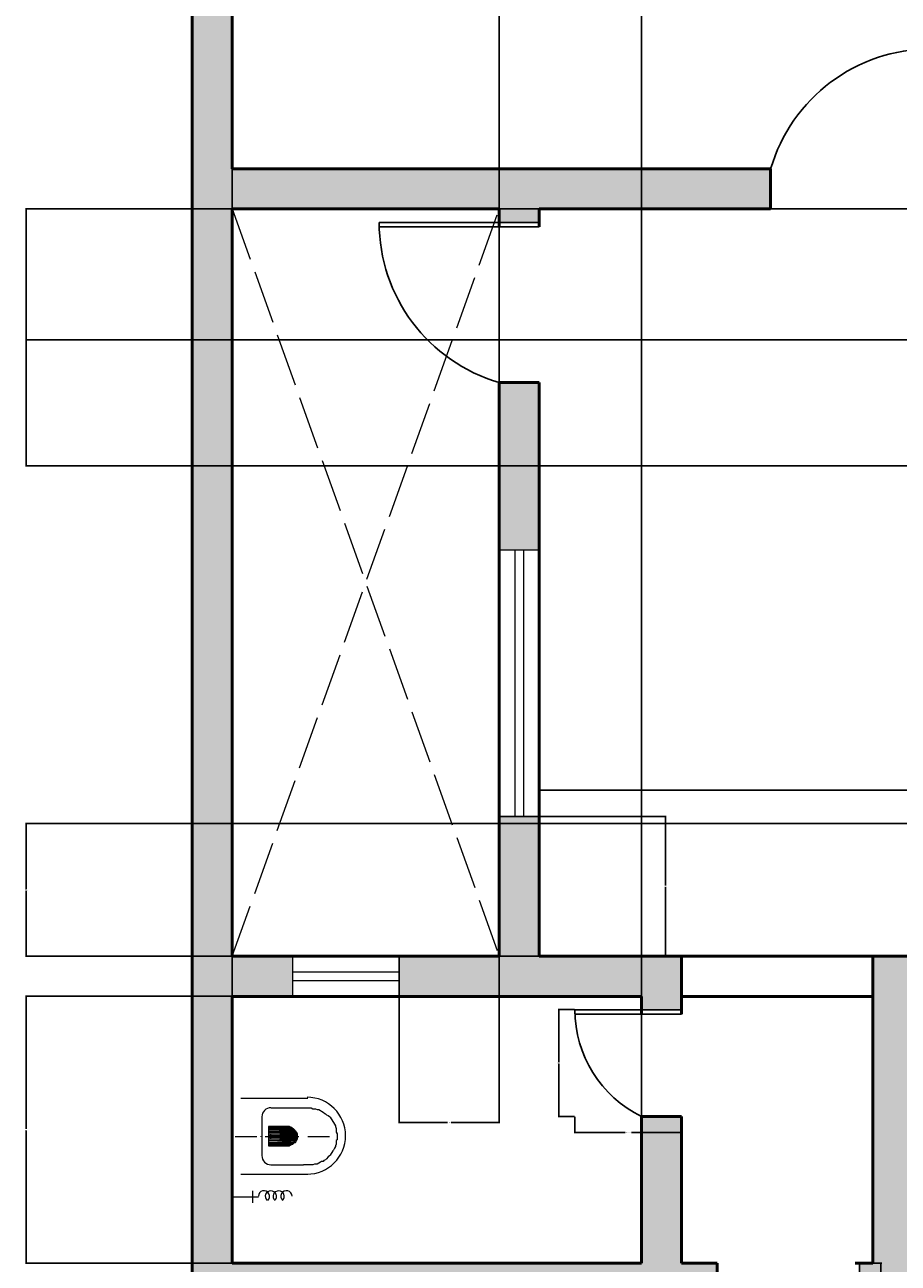
# Model space of a CAD drawing. Units: inches. Extents: x 383 to 970, y 275 to 1088.
# Tile 5 of 11: x 383 to 579, y 546 to 825. Entities that reach past the tile are written whole.
import ezdxf

# ---------------------------------------------------------------- set-up
doc = ezdxf.new("R2010")
doc.units = ezdxf.units.IN
doc.header["$MEASUREMENT"] = 0
doc.linetypes.add('ACAD_ISO02W100', pattern=[15, 12, -3])
for name, color, linetype, lineweight in [('A-ANNO-DIMS', 2, 'Continuous', 18), ('A-DOOR', 3, 'Continuous', 25), ('A-FLOR-FIXT', 8, 'Continuous', 18), ('A-FLOR-OPEN', 8, 'ACAD_ISO02W100', 13), ('A-GLAZ', 4, 'Continuous', 18), ('A-WALL', 7, 'Continuous', 50)]:
    doc.layers.add(name, color=color, linetype=linetype, lineweight=lineweight)
doc.layers.add('A-WALL-PATT', color=251, linetype='Continuous', lineweight=13, true_color=0x636466)
doc.styles.get("Standard").update_dxf_attribs({"font": 'arial.ttf'})
doc.dimstyles.get("Standard").update_dxf_attribs({"dimtxt": 0.18, "dimasz": 0.18, "dimexe": 0.18, "dimexo": 0.0625, "dimgap": 0.09, "dimtad": 0, "dimtih": 1, "dimtoh": 1, "dimdec": 4, "dimzin": 0, "dimdsep": 46, "dimtxsty": 'Standard', "dimcen": 0.09, "dimadec": 0, "dimazin": 0, "dimtfac": 1, "dimtdec": 4, "dimtofl": 0, "dimtmove": 0, "dimatfit": 3, "dimfxl": 1, "dimtolj": 1, "dimtzin": 0, "dimarcsym": 0})

# ---------------------------------------------------------------- blocks, each defined once
blk = doc.blocks.new('WC-PLAN')
h = blk.add_hatch(color=256)
h.paths.add_polyline_path([(8.12, 16.94), (13.2, 16.94), (8.12, 17.17)])
h.paths.add_polyline_path([(13.2, 16.94), (8.12, 17.17), (12.82, 17.17)])
h.paths.add_polyline_path([(8.12, 17.17), (12.82, 17.17), (12.44, 17.17)])
h = blk.add_hatch(color=256)
h.paths.add_polyline_path([(8.12, 16.71), (13.58, 16.71), (8.12, 16.94)])
h.paths.add_polyline_path([(13.58, 16.71), (8.12, 16.94), (13.2, 16.94)])
h = blk.add_hatch(color=256)
h.paths.add_polyline_path([(8.12, 16.56), (13.81, 16.56), (8.12, 16.71)])
h.paths.add_polyline_path([(13.81, 16.56), (8.12, 16.71), (13.58, 16.71)])
h = blk.add_hatch(color=256)
h.paths.add_polyline_path([(8.12, 16.18), (14.19, 16.18), (8.12, 16.56)])
h.paths.add_polyline_path([(14.19, 16.18), (8.12, 16.56), (13.81, 16.56)])
h = blk.add_hatch(color=256)
h.paths.add_polyline_path([(8.12, 15.95), (14.34, 15.95), (8.12, 16.18)])
h.paths.add_polyline_path([(14.34, 15.95), (8.12, 16.18), (14.19, 16.18)])
h = blk.add_hatch(color=256)
h.paths.add_polyline_path([(8.12, 15.57), (14.56, 15.57), (8.12, 15.95)])
h.paths.add_polyline_path([(14.56, 15.57), (8.12, 15.95), (14.34, 15.95)])
h = blk.add_hatch(color=256)
h.paths.add_polyline_path([(8.12, 15.19), (14.56, 15.19), (8.12, 15.57)])
h.paths.add_polyline_path([(14.56, 15.19), (8.12, 15.57), (14.56, 15.57)])
h = blk.add_hatch(color=256)
h.paths.add_polyline_path([(8.12, 14.81), (14.56, 14.81), (8.12, 15.19)])
h.paths.add_polyline_path([(14.56, 14.81), (8.12, 15.19), (14.56, 15.19)])
h = blk.add_hatch(color=256)
h.paths.add_polyline_path([(8.12, 14.44), (14.56, 14.44), (8.12, 14.81)])
h.paths.add_polyline_path([(14.56, 14.44), (8.12, 14.81), (14.56, 14.81)])
h = blk.add_hatch(color=256)
h.paths.add_polyline_path([(8.12, 14.06), (14.34, 14.06), (8.12, 14.44)])
h.paths.add_polyline_path([(14.34, 14.06), (8.12, 14.44), (14.56, 14.44)])
h = blk.add_hatch(color=256)
h.paths.add_polyline_path([(8.12, 13.6), (14.19, 13.6), (8.12, 14.06)])
h.paths.add_polyline_path([(14.19, 13.6), (8.12, 14.06), (14.34, 14.06)])
h = blk.add_hatch(color=256)
h.paths.add_polyline_path([(8.12, 13.45), (13.81, 13.45), (8.12, 13.6)])
h.paths.add_polyline_path([(13.81, 13.45), (8.12, 13.6), (14.19, 13.6)])
h = blk.add_hatch(color=256)
h.paths.add_polyline_path([(8.12, 13.22), (13.58, 13.22), (8.12, 13.45)])
h.paths.add_polyline_path([(13.58, 13.22), (8.12, 13.45), (13.81, 13.45)])
h = blk.add_hatch(color=256)
h.paths.add_polyline_path([(8.12, 13.07), (13.2, 13.07), (8.12, 13.22)])
h.paths.add_polyline_path([(13.2, 13.07), (8.12, 13.22), (13.58, 13.22)])
h = blk.add_hatch(color=256)
h.paths.add_polyline_path([(8.12, 12.84), (12.82, 12.84), (8.12, 13.07)])
h.paths.add_polyline_path([(12.82, 12.84), (8.12, 13.07), (13.2, 13.07)])
for points in [[(1.9, 23.54), (16.92, 23.54), (16.92, 23.54)], [(8.72, 21.41), (15.93, 21.41), (15.93, 21.41)], [(15.93, 21.41), (16.69, 21.41), (17.3, 21.41), (17.67, 21.41), (18.05, 21.19), (18.43, 21.19), (18.66, 21.19), (19.04, 21.03), (19.42, 21.03), (19.8, 20.81), (20.03, 20.66), (20.41, 20.43), (20.56, 20.28), (20.94, 20.05), (21.16, 19.82), (21.54, 19.67), (21.77, 19.44), (21.92, 19.29), (22.15, 18.91), (22.3, 18.68), (22.53, 18.3), (22.68, 18.08), (22.91, 17.7), (23.14, 17.32), (23.14, 17.17), (23.29, 16.71), (23.29, 16.33), (23.29, 15.95), (23.52, 15.57), (23.52, 14.97), (23.52, 14.21), (23.29, 14.06), (23.29, 13.6), (23.29, 13.22), (23.14, 12.84), (23.14, 12.69), (22.91, 12.31), (22.68, 11.86), (22.53, 11.7), (22.3, 11.32), (22.15, 11.1), (21.92, 10.72), (21.77, 10.57), (21.54, 10.34), (21.16, 9.96), (20.94, 9.73), (20.56, 9.58), (20.41, 9.35), (20.03, 9.35), (19.8, 9.2), (19.42, 8.97), (19.04, 8.75), (18.66, 8.75), (18.43, 8.75), (18.05, 8.59), (17.67, 8.59), (17.3, 8.59), (16.69, 8.59), (15.93, 8.59)], [(6.6, 19.29), (6.6, 10.57), (6.6, 10.57)], [(8.12, 17.17), (8.12, 12.84), (8.12, 12.84)], [(8.12, 17.17), (12.44, 17.17), (12.44, 17.17)], [(0.61, 14.97), (5.46, 14.97), (5.46, 14.97)], [(6.37, 14.97), (6.37, 15.04), (6.37, 15.04)], [(7.36, 14.97), (14.94, 14.97), (14.94, 14.97)], [(8.57, 15.42), (8.5, 15.42), (8.5, 15.42)], [(8.57, 14.97), (8.5, 15.04), (8.5, 15.04)], [(8.57, 14.59), (8.5, 14.59), (8.5, 14.59)], [(8.57, 15.42), (8.57, 15.19), (8.57, 14.97)], [(8.57, 14.97), (8.57, 14.81), (8.57, 14.59)], [(16.92, 14.97), (21.77, 14.97), (21.77, 14.97)], [(8.12, 12.84), (12.44, 12.84), (12.44, 12.84)], [(8.72, 8.59), (15.93, 8.59), (15.93, 8.59)], [(1.9, 6.47), (16.92, 6.47), (16.92, 6.47)], [(0, 1.37), (5.84, 1.37), (5.84, 1.37)], [(4.48, 2.73), (4.48, 0), (4.48, 0)]]:
    blk.add_lwpolyline(points)
for points in [[(8.12, 16.94), (13.2, 16.94), (8.12, 17.17)], [(13.2, 16.94), (8.12, 17.17), (12.82, 17.17)], [(8.12, 17.17), (12.82, 17.17), (12.44, 17.17)], [(12.82, 17.17), (8.12, 17.17), (8.12, 17.17)], [(8.12, 16.71), (13.58, 16.71), (8.12, 16.94)], [(13.58, 16.71), (8.12, 16.94), (13.2, 16.94)], [(8.12, 16.56), (13.81, 16.56), (8.12, 16.71)], [(13.81, 16.56), (8.12, 16.71), (13.58, 16.71)], [(8.12, 16.18), (14.19, 16.18), (8.12, 16.56)], [(14.19, 16.18), (8.12, 16.56), (13.81, 16.56)], [(8.12, 15.95), (14.34, 15.95), (8.12, 16.18)], [(14.34, 15.95), (8.12, 16.18), (14.19, 16.18)], [(8.12, 15.57), (14.56, 15.57), (8.12, 15.95)], [(14.56, 15.57), (8.12, 15.95), (14.34, 15.95)], [(8.12, 15.19), (14.56, 15.19), (8.12, 15.57)], [(14.56, 15.19), (8.12, 15.57), (14.56, 15.57)], [(8.12, 14.81), (14.56, 14.81), (8.12, 15.19)], [(14.56, 14.81), (8.12, 15.19), (14.56, 15.19)], [(8.12, 14.44), (14.56, 14.44), (8.12, 14.81)], [(14.56, 14.44), (8.12, 14.81), (14.56, 14.81)], [(8.12, 14.06), (14.34, 14.06), (8.12, 14.44)], [(14.34, 14.06), (8.12, 14.44), (14.56, 14.44)], [(8.12, 13.6), (14.19, 13.6), (8.12, 14.06)], [(14.19, 13.6), (8.12, 14.06), (14.34, 14.06)], [(8.12, 13.45), (13.81, 13.45), (8.12, 13.6)], [(13.81, 13.45), (8.12, 13.6), (14.19, 13.6)], [(8.12, 13.22), (13.58, 13.22), (8.12, 13.45)], [(13.58, 13.22), (8.12, 13.45), (13.81, 13.45)], [(8.12, 13.07), (13.2, 13.07), (8.12, 13.22)], [(13.2, 13.07), (8.12, 13.22), (13.58, 13.22)], [(8.12, 12.84), (12.82, 12.84), (8.12, 13.07)], [(12.82, 12.84), (8.12, 13.07), (13.2, 13.07)], [(8.12, 12.84), (12.44, 12.84)], [(12.44, 12.84), (8.12, 12.84), (12.82, 12.84)]]:
    blk.add_lwpolyline(points, close=True)
for points, knots in [([(16.76, 6.47), (21.54, 6.47), (25.41, 10.34), (25.41, 15.12), (25.41, 15.12), (25.41, 19.9), (21.54, 23.77), (16.76, 23.77)], [0, 0, 0, 0, 0.125, 0.125, 0.125, 0.125001, 1, 1, 1, 1]), ([(12.29, 13.07), (13.43, 13.07), (14.34, 13.98), (14.34, 15.12), (14.34, 15.12), (14.34, 16.26), (13.43, 17.17), (12.29, 17.17)], [0, 0, 0, 0, 0.125, 0.125, 0.125, 0.125001, 1, 1, 1, 1]), ([(7.97, 0.53), (8.34, 0.91), (8.5, 1.59), (8.19, 2.05), (8.19, 2.05), (7.89, 2.58), (7.36, 2.88), (6.75, 2.73), (6.75, 2.73), (6.22, 2.58), (5.84, 2.05), (5.84, 1.52)], [0, 0, 0, 0, 0.083333, 0.083333, 0.083333, 0.083334, 0.166667, 0.166667, 0.166667, 0.166668, 1, 1, 1, 1]), ([(13.43, 1.52), (13.43, 2.05), (12.97, 2.58), (12.44, 2.73), (12.44, 2.73), (11.91, 2.88), (11.3, 2.58), (11, 2.12), (11, 2.12), (10.77, 1.59), (10.85, 0.99), (11.23, 0.61)], [0, 0, 0, 0, 0.083333, 0.083333, 0.083333, 0.083334, 0.166667, 0.166667, 0.166667, 0.166668, 1, 1, 1, 1]), ([(9.48, 0.61), (9.86, 0.91), (10.01, 1.52), (9.79, 1.97), (9.79, 1.97), (9.63, 2.43), (9.1, 2.73), (8.65, 2.73), (8.65, 2.73), (8.12, 2.73), (7.66, 2.43), (7.43, 1.97), (7.43, 1.97), (7.28, 1.44), (7.43, 0.91), (7.81, 0.53)], [0, 0, 0, 0, 0.0625, 0.0625, 0.0625, 0.062501, 0.125, 0.125, 0.125, 0.125001, 0.1875, 0.1875, 0.1875, 0.187501, 1, 1, 1, 1]), ([(11.23, 0.53), (11.61, 0.91), (11.76, 1.44), (11.53, 1.97), (11.53, 1.97), (11.38, 2.43), (10.92, 2.73), (10.39, 2.73), (10.39, 2.73), (9.86, 2.73), (9.41, 2.43), (9.18, 1.97), (9.18, 1.97), (9.03, 1.44), (9.18, 0.91), (9.56, 0.53)], [0, 0, 0, 0, 0.0625, 0.0625, 0.0625, 0.062501, 0.125, 0.125, 0.125, 0.125001, 0.1875, 0.1875, 0.1875, 0.187501, 1, 1, 1, 1])]:
    blk.add_open_spline(points, degree=3, knots=knots)
for points in [[(8.65, 21.41), (7.51, 21.41), (6.6, 20.5), (6.6, 19.37)], [(6.6, 10.64), (6.6, 9.5), (7.51, 8.59), (8.65, 8.59)]]:
    blk.add_open_spline(points, degree=3)
blk = doc.blocks.new('DOOR-LEAF-36IN')
for p, q in [((0, 0), (0, 36)), ((1, 36), (1, 0)), ((0, 0), (1, 0))]:
    blk.add_line(p, q)
blk.add_arc((0, -1.5), 37.5, 16.2602, 90)
blk = doc.blocks.new('DOOR-LEAF-24IN')
for p, q in [((23, 24), (23, 0)), ((24, 0), (24, 24)), ((24, 0), (23, 0))]:
    blk.add_line(p, q)
blk.add_arc((24, -2.7), 26.7, 90, 154.0108)
blk = doc.blocks.new('WIN-VENT-24IN')
for p, q in [((0, 0), (0, 24)), ((3.5, 0), (3.5, 24)), ((5.5, 24), (5.5, 0)), ((9, 24), (9, 0))]:
    blk.add_line(p, q)
blk = doc.blocks.new('WIN-60IN')
for p, q in [((60, 9), (0, 9)), ((60, 5.5), (0, 5.5)), ((0, 3.5), (60, 3.5)), ((0, 0), (60, 0))]:
    blk.add_line(p, q)
blk = doc.blocks.new('*D15')
at = {"layer": 'A-ANNO-DIMS', "color": 0, "lineweight": -2, "transparency": 16777216}
for p, q in [((570.3, 546.14), (575.22, 546.14)), ((575.04, 545.96), (575.04, 530.32)), ((575.04, 514.32), (575.04, 529.95)), ((570.3, 514.14), (575.22, 514.14))]:
    blk.add_line(p, q, dxfattribs=at)
at = {"layer": 'A-ANNO-DIMS', "color": 0, "transparency": 16777216}
for points in [[(575.01, 545.96), (575.07, 545.96), (575.04, 546.14)], [(575.01, 514.32), (575.07, 514.32), (575.04, 514.14)]]:
    blk.add_solid(points, dxfattribs=at)
at = {"layer": 'Defpoints', "color": 0, "transparency": 16777216}
for p in [(570.24, 546.14), (575.04, 546.14), (570.24, 514.14)]:
    blk.add_point(p, dxfattribs=at)
at = {"layer": 'A-ANNO-DIMS', "color": 0, "transparency": 16777216, "insert": (575.04, 530.14), "char_height": 0.18, "attachment_point": 5}
blk.add_mtext('\\A1;D2 32 TYP.', dxfattribs=at)
blk = doc.blocks.new('*D17')
at = {"layer": 'A-ANNO-DIMS', "color": 0, "lineweight": -2, "transparency": 16777216}
for p, q in [((506.24, 579.07), (506.24, 575.36)), ((530.24, 579.07), (530.24, 575.36)), ((506.42, 575.54), (517.52, 575.54)), ((530.06, 575.54), (518.96, 575.54))]:
    blk.add_line(p, q, dxfattribs=at)
at = {"layer": 'A-ANNO-DIMS', "color": 0, "transparency": 16777216}
for points in [[(506.42, 575.57), (506.42, 575.51), (506.24, 575.54)], [(530.06, 575.57), (530.06, 575.51), (530.24, 575.54)]]:
    blk.add_solid(points, dxfattribs=at)
at = {"layer": 'Defpoints', "color": 0, "transparency": 16777216}
for p in [(506.24, 579.14), (530.24, 579.14), (506.24, 575.54)]:
    blk.add_point(p, dxfattribs=at)
at = {"layer": 'A-ANNO-DIMS', "color": 0, "transparency": 16777216, "insert": (518.24, 575.54), "char_height": 0.18, "attachment_point": 5}
blk.add_mtext('\\A1;D3 24 TYP.', dxfattribs=at)
blk = doc.blocks.new('*D18')
at = {"layer": 'A-ANNO-DIMS', "color": 0, "lineweight": -2, "transparency": 16777216}
for p, q in [((506.18, 603.14), (502.46, 603.14)), ((502.64, 602.96), (502.64, 591.32)), ((502.64, 579.32), (502.64, 590.96)), ((506.18, 579.14), (502.46, 579.14))]:
    blk.add_line(p, q, dxfattribs=at)
at = {"layer": 'A-ANNO-DIMS', "color": 0, "transparency": 16777216}
for points in [[(502.61, 602.96), (502.67, 602.96), (502.64, 603.14)], [(502.61, 579.32), (502.67, 579.32), (502.64, 579.14)]]:
    blk.add_solid(points, dxfattribs=at)
at = {"layer": 'Defpoints', "color": 0, "transparency": 16777216}
for p in [(502.64, 603.14), (506.24, 603.14), (506.24, 579.14)]:
    blk.add_point(p, dxfattribs=at)
at = {"layer": 'A-ANNO-DIMS', "color": 0, "transparency": 16777216, "insert": (502.64, 591.14), "char_height": 0.18, "attachment_point": 5}
blk.add_mtext('\\A1;24 TYP.', dxfattribs=at)
blk = doc.blocks.new('*D39')
at = {"layer": 'A-ANNO-DIMS', "color": 0, "lineweight": -2, "transparency": 16777216}
for p, q in [((429.18, 606.14), (382.71, 606.14)), ((382.89, 605.96), (382.89, 576.32)), ((382.89, 546.32), (382.89, 575.95)), ((429.18, 546.14), (382.71, 546.14))]:
    blk.add_line(p, q, dxfattribs=at)
at = {"layer": 'A-ANNO-DIMS', "color": 0, "transparency": 16777216}
for points in [[(382.86, 605.96), (382.92, 605.96), (382.89, 606.14)], [(382.86, 546.32), (382.92, 546.32), (382.89, 546.14)]]:
    blk.add_solid(points, dxfattribs=at)
at = {"layer": 'Defpoints', "color": 0, "transparency": 16777216}
for p in [(382.89, 606.14), (429.24, 606.14), (429.24, 546.14)]:
    blk.add_point(p, dxfattribs=at)
at = {"layer": 'A-ANNO-DIMS', "color": 0, "transparency": 16777216, "insert": (382.89, 576.14), "char_height": 0.18, "attachment_point": 5}
blk.add_mtext('\\A1;60', dxfattribs=at)
blk = doc.blocks.new('*D48')
at = {"layer": 'A-ANNO-DIMS', "color": 0, "lineweight": -2, "transparency": 16777216}
for p, q in [((429.24, 546.2), (429.24, 1087.67)), ((429.42, 1087.49), (475.02, 1087.49)), ((521.06, 1087.49), (475.46, 1087.49)), ((521.24, 546.2), (521.24, 1087.67))]:
    blk.add_line(p, q, dxfattribs=at)
at = {"layer": 'A-ANNO-DIMS', "color": 0, "transparency": 16777216}
for points in [[(429.42, 1087.52), (429.42, 1087.46), (429.24, 1087.49)], [(521.06, 1087.52), (521.06, 1087.46), (521.24, 1087.49)]]:
    blk.add_solid(points, dxfattribs=at)
at = {"layer": 'Defpoints', "color": 0, "transparency": 16777216}
for p in [(521.24, 1087.49), (429.24, 546.14), (521.24, 546.14)]:
    blk.add_point(p, dxfattribs=at)
at = {"layer": 'A-ANNO-DIMS', "color": 0, "transparency": 16777216, "insert": (475.24, 1087.49), "char_height": 0.18, "attachment_point": 5}
blk.add_mtext('\\A1;92', dxfattribs=at)
blk = doc.blocks.new('*D49')
at = {"layer": 'A-ANNO-DIMS', "color": 0, "lineweight": -2, "transparency": 16777216}
for p, q in [((429.24, 615.2), (429.24, 1087.67)), ((429.42, 1087.49), (459.02, 1087.49)), ((489.06, 1087.49), (459.46, 1087.49)), ((489.24, 615.2), (489.24, 1087.67))]:
    blk.add_line(p, q, dxfattribs=at)
at = {"layer": 'A-ANNO-DIMS', "color": 0, "transparency": 16777216}
for points in [[(429.42, 1087.52), (429.42, 1087.46), (429.24, 1087.49)], [(489.06, 1087.52), (489.06, 1087.46), (489.24, 1087.49)]]:
    blk.add_solid(points, dxfattribs=at)
at = {"layer": 'Defpoints', "color": 0, "transparency": 16777216}
for p in [(489.24, 1087.49), (429.24, 615.14), (489.24, 615.14)]:
    blk.add_point(p, dxfattribs=at)
at = {"layer": 'A-ANNO-DIMS', "color": 0, "transparency": 16777216, "insert": (459.24, 1087.49), "char_height": 0.18, "attachment_point": 5}
blk.add_mtext('\\A1;60', dxfattribs=at)
blk = doc.blocks.new('*D53')
at = {"layer": 'A-ANNO-DIMS', "color": 0, "lineweight": -2, "transparency": 16777216}
for p, q in [((814.18, 783.14), (382.71, 783.14)), ((382.89, 782.96), (382.89, 768.63)), ((382.89, 753.94), (382.89, 768.27)), ((814.18, 753.76), (382.71, 753.76))]:
    blk.add_line(p, q, dxfattribs=at)
at = {"layer": 'A-ANNO-DIMS', "color": 0, "transparency": 16777216}
for points in [[(382.86, 782.96), (382.92, 782.96), (382.89, 783.14)], [(382.86, 753.94), (382.92, 753.94), (382.89, 753.76)]]:
    blk.add_solid(points, dxfattribs=at)
at = {"layer": 'Defpoints', "color": 0, "transparency": 16777216}
for p in [(814.24, 783.14), (382.89, 753.76), (814.24, 753.76)]:
    blk.add_point(p, dxfattribs=at)
at = {"layer": 'A-ANNO-DIMS', "color": 0, "transparency": 16777216, "insert": (382.89, 768.45), "char_height": 0.18, "attachment_point": 5}
blk.add_mtext('\\A1;29.38', dxfattribs=at)
blk = doc.blocks.new('*D54')
at = {"layer": 'A-ANNO-DIMS', "color": 0, "lineweight": -2, "transparency": 16777216}
for p, q in [((814.18, 644.96), (382.71, 644.96)), ((382.89, 644.78), (382.89, 630.23)), ((382.89, 615.32), (382.89, 629.86)), ((814.18, 615.14), (382.71, 615.14))]:
    blk.add_line(p, q, dxfattribs=at)
at = {"layer": 'A-ANNO-DIMS', "color": 0, "transparency": 16777216}
for points in [[(382.86, 644.78), (382.92, 644.78), (382.89, 644.96)], [(382.86, 615.32), (382.92, 615.32), (382.89, 615.14)]]:
    blk.add_solid(points, dxfattribs=at)
at = {"layer": 'Defpoints', "color": 0, "transparency": 16777216}
for p in [(382.89, 644.96), (814.24, 644.96), (814.24, 615.14)]:
    blk.add_point(p, dxfattribs=at)
at = {"layer": 'A-ANNO-DIMS', "color": 0, "transparency": 16777216, "insert": (382.89, 630.05), "char_height": 0.18, "attachment_point": 5}
blk.add_mtext('\\A1;29.82', dxfattribs=at)
blk = doc.blocks.new('*D56')
at = {"layer": 'A-ANNO-DIMS', "color": 0, "lineweight": -2, "transparency": 16777216}
for p, q in [((805.18, 783.14), (382.71, 783.14)), ((382.89, 782.96), (382.89, 754.44)), ((382.89, 725.56), (382.89, 754.08)), ((805.18, 725.38), (382.71, 725.38))]:
    blk.add_line(p, q, dxfattribs=at)
at = {"layer": 'A-ANNO-DIMS', "color": 0, "transparency": 16777216}
for points in [[(382.86, 782.96), (382.92, 782.96), (382.89, 783.14)], [(382.86, 725.56), (382.92, 725.56), (382.89, 725.38)]]:
    blk.add_solid(points, dxfattribs=at)
at = {"layer": 'Defpoints', "color": 0, "transparency": 16777216}
for p in [(382.89, 783.14), (805.24, 783.14), (805.24, 725.38)]:
    blk.add_point(p, dxfattribs=at)
at = {"layer": 'A-ANNO-DIMS', "color": 0, "transparency": 16777216, "insert": (382.89, 754.26), "char_height": 0.18, "attachment_point": 5}
blk.add_mtext('\\A1;57.76', dxfattribs=at)
blk = doc.blocks.new('*D64')
at = {"layer": 'A-ANNO-DIMS', "color": 0, "lineweight": -2, "transparency": 16777216}
for p, q in [((489.3, 646.54), (526.77, 646.54)), ((526.59, 646.36), (526.59, 631.02)), ((526.59, 615.32), (526.59, 630.65)), ((489.3, 615.14), (526.77, 615.14))]:
    blk.add_line(p, q, dxfattribs=at)
at = {"layer": 'A-ANNO-DIMS', "color": 0, "transparency": 16777216}
for points in [[(526.56, 646.36), (526.62, 646.36), (526.59, 646.54)], [(526.56, 615.32), (526.62, 615.32), (526.59, 615.14)]]:
    blk.add_solid(points, dxfattribs=at)
at = {"layer": 'Defpoints', "color": 0, "transparency": 16777216}
for p in [(489.24, 646.54), (489.24, 615.14), (526.59, 615.14)]:
    blk.add_point(p, dxfattribs=at)
at = {"layer": 'A-ANNO-DIMS', "color": 0, "transparency": 16777216, "insert": (526.59, 630.84), "char_height": 0.18, "attachment_point": 5}
blk.add_mtext('\\A1;31.4', dxfattribs=at)
blk = doc.blocks.new('*D67')
at = {"layer": 'A-ANNO-DIMS', "color": 0, "lineweight": -2, "transparency": 16777216}
for p, q in [((498.24, 615.2), (498.24, 652.67)), ((498.42, 652.49), (651.45, 652.49)), ((805.06, 652.49), (652.03, 652.49)), ((805.24, 615.2), (805.24, 652.67))]:
    blk.add_line(p, q, dxfattribs=at)
at = {"layer": 'A-ANNO-DIMS', "color": 0, "transparency": 16777216}
for points in [[(498.42, 652.52), (498.42, 652.46), (498.24, 652.49)], [(805.06, 652.52), (805.06, 652.46), (805.24, 652.49)]]:
    blk.add_solid(points, dxfattribs=at)
at = {"layer": 'Defpoints', "color": 0, "transparency": 16777216}
for p in [(805.24, 652.49), (498.24, 615.14), (805.24, 615.14)]:
    blk.add_point(p, dxfattribs=at)
at = {"layer": 'A-ANNO-DIMS', "color": 0, "transparency": 16777216, "insert": (651.74, 652.49), "char_height": 0.18, "attachment_point": 5}
blk.add_mtext('\\A1;307', dxfattribs=at)
blk = doc.blocks.new('*D70')
at = {"layer": 'A-ANNO-DIMS', "color": 0, "lineweight": -2, "transparency": 16777216}
for p, q in [((466.77, 615.07), (466.77, 577.61)), ((489.24, 615.07), (489.24, 577.61)), ((466.95, 577.79), (477.61, 577.79)), ((489.06, 577.79), (478.4, 577.79))]:
    blk.add_line(p, q, dxfattribs=at)
at = {"layer": 'A-ANNO-DIMS', "color": 0, "transparency": 16777216}
for points in [[(466.95, 577.82), (466.95, 577.76), (466.77, 577.79)], [(489.06, 577.82), (489.06, 577.76), (489.24, 577.79)]]:
    blk.add_solid(points, dxfattribs=at)
at = {"layer": 'Defpoints', "color": 0, "transparency": 16777216}
for p in [(466.77, 615.14), (489.24, 615.14), (466.77, 577.79)]:
    blk.add_point(p, dxfattribs=at)
at = {"layer": 'A-ANNO-DIMS', "color": 0, "transparency": 16777216, "insert": (478.01, 577.79), "char_height": 0.18, "attachment_point": 5}
blk.add_mtext('\\A1;22.47', dxfattribs=at)

msp = doc.modelspace()

# ---------------------------------------------------------------- hatches: boundary and pattern name
at = {"layer": 'A-WALL-PATT'}
h = msp.add_hatch(color=256, dxfattribs=at)
h.dxf.hatch_style = 1
h.paths.add_polyline_path([(651.24, 321.1365), (651.24, 417.1365), (735.24, 417.1365), (735.24, 491.9233), (726.24, 491.9233), (726.24, 426.1365), (582.24, 426.1365), (582.24, 606.1365), (687.24, 606.1365), (687.24, 615.1365), (573.24, 615.1365), (573.24, 546.1365), (570.24, 546.1365), (570.24, 537.1365), (573.24, 537.1365), (573.24, 414.1365), (582.24, 414.1365), (582.24, 417.1365), (642.24, 417.1365), (642.24, 321.1365), (621.6203, 321.1365), (621.6203, 312.1365), (651.24, 312.1365)], flags=17)
h.paths.add_polyline_path([(597.6203, 321.1365), (582.24, 321.1365), (582.24, 390.1365), (573.24, 390.1365), (573.24, 321.1365), (570.24, 321.1365), (570.24, 312.1365), (573.24, 312.1365), (597.6203, 312.1365)], flags=16)
h.paths.add_polyline_path([(534.24, 321.1365), (500.8868, 321.1365), (500.8868, 312.1365), (534.24, 312.1365)], flags=17)
h.paths.add_polyline_path([(735.24, 606.1365), (738.24, 606.1365), (738.24, 615.1365), (723.24, 615.1365), (723.24, 606.1365), (726.24, 606.1365), (726.24, 551.9233), (735.24, 551.9233)], flags=17)
h.paths.add_polyline_path([(848.0899, 615.1365), (814.24, 615.1365), (814.24, 689.38), (805.24, 689.38), (805.24, 615.1365), (802.24, 615.1365), (802.24, 606.1365), (848.0899, 606.1365)], flags=17)
h.paths.add_polyline_path([(530.24, 615.1365), (498.24, 615.1365), (498.24, 646.5351), (489.24, 646.5351), (489.24, 615.1365), (466.771, 615.1365), (466.771, 606.1365), (521.24, 606.1365), (521.24, 603.1365), (530.24, 603.1365), (530.24, 606.1365)], flags=17)
h.paths.add_polyline_path([(498.24, 744.1365), (489.24, 744.1365), (489.24, 706.5351), (498.24, 706.5351)], flags=17)
h.paths.add_polyline_path([(715.24, 792.1365), (598.24, 792.1365), (598.24, 972.1365), (636.5058, 972.1365), (636.5058, 981.1365), (589.24, 981.1365), (589.24, 972.1365), (589.24, 792.1365), (586.24, 792.1365), (586.24, 783.1365), (589.24, 783.1365), (715.24, 783.1365)], flags=17)
h.paths.add_polyline_path([(763.24, 981.1365), (696.5058, 981.1365), (696.5058, 972.1365), (754.24, 972.1365), (754.24, 792.1365), (751.24, 792.1365), (751.24, 783.1365), (754.24, 783.1365), (764.24, 783.1365), (764.24, 792.1365), (763.24, 792.1365)], flags=17)
h.paths.add_polyline_path([(815.24, 1001.9492), (806.24, 1001.9492), (806.24, 972.1365), (818.24, 972.1365), (818.24, 981.1365), (815.24, 981.1365)], flags=17)
h.paths.add_polyline_path([(546.24, 1004.0336), (537.24, 1004.0336), (537.24, 981.1365), (534.24, 981.1365), (534.24, 972.1365), (537.24, 972.1365), (546.24, 972.1365), (546.24, 981.1365)], flags=17)
h.paths.add_polyline_path([(884.0899, 606.1365), (932.24, 606.1365), (932.24, 1050.1365), (420.24, 1050.1365), (420.24, 312.1365), (440.8868, 312.1365), (440.8868, 321.1365), (429.24, 321.1365), (429.24, 537.1365), (538.24, 537.1365), (538.24, 546.1365), (530.24, 546.1365), (530.24, 579.1365), (521.24, 579.1365), (521.24, 546.1365), (429.24, 546.1365), (429.24, 606.1365), (442.771, 606.1365), (442.771, 615.1365), (429.24, 615.1365), (429.24, 783.1365), (489.24, 783.1365), (489.24, 780.1365), (498.24, 780.1365), (498.24, 783.1365), (550.24, 783.1365), (550.24, 792.1365), (429.24, 792.1365), (429.24, 972.1365), (510.24, 972.1365), (510.24, 981.1365), (429.24, 981.1365), (429.24, 1041.1365), (537.24, 1041.1365), (537.24, 1028.0336), (546.24, 1028.0336), (546.24, 1041.1365), (806.24, 1041.1365), (806.24, 1025.9492), (815.24, 1025.9492), (815.24, 1041.1365), (923.24, 1041.1365), (923.24, 981.1365), (842.24, 981.1365), (842.24, 972.1365), (923.24, 972.1365), (923.24, 792.1365), (800.24, 792.1365), (800.24, 783.1365), (805.24, 783.1365), (805.24, 725.38), (814.24, 725.38), (814.24, 783.1365), (923.24, 783.1365), (923.24, 615.1365), (884.0899, 615.1365)])

# ---------------------------------------------------------------- linework, layer by layer
at = {"layer": 'A-DOOR'}
for p, q in [((462.24, 780.1365), (498.24, 780.1365)), ((506.24, 603.1365), (530.24, 603.1365)), ((570.24, 514.1365), (570.24, 546.1365))]:
    msp.add_line(p, q, dxfattribs=at)
at = {"layer": 'A-FLOR-OPEN'}
for p, q in [((429.24, 615.1365), (489.24, 783.1365)), ((429.24, 783.1365), (489.24, 615.1365))]:
    msp.add_line(p, q, dxfattribs=at)
at = {"layer": 'A-GLAZ'}
for p, q in [((489.24, 706.5351), (498.24, 706.5351)), ((498.24, 646.5351), (489.24, 646.5351)), ((442.771, 615.1365), (442.771, 606.1365)), ((466.771, 606.1365), (466.771, 615.1365))]:
    msp.add_line(p, q, dxfattribs=at)
at = {"layer": 'A-WALL'}
for p, q in [((420.24, 1050.1365), (420.24, 312.1365)), ((429.24, 972.1365), (429.24, 792.1365)), ((429.24, 792.1365), (550.24, 792.1365)), ((550.24, 783.1365), (550.24, 792.1365)), ((429.24, 783.1365), (489.24, 783.1365)), ((429.24, 783.1365), (429.24, 615.1365)), ((489.24, 783.1365), (489.24, 779.1365)), ((498.24, 783.1365), (498.24, 779.1365)), ((498.24, 783.1365), (498.24, 780.1365)), ((498.24, 783.1365), (550.24, 783.1365)), ((498.24, 744.1365), (489.24, 744.1365)), ((489.24, 744.1365), (489.24, 615.1365)), ((498.24, 744.1365), (498.24, 615.1365)), ((429.24, 615.1365), (489.24, 615.1365)), ((498.24, 615.1365), (687.24, 615.1365)), ((530.24, 615.1365), (530.24, 602.1365)), ((573.24, 615.1365), (573.24, 546.1365)), ((429.24, 606.1365), (521.24, 606.1365)), ((429.24, 606.1365), (429.24, 546.1365)), ((521.24, 606.1365), (521.24, 602.1365)), ((530.24, 606.1365), (530.24, 603.1365)), ((530.24, 606.1365), (573.24, 606.1365)), ((530.24, 579.1365), (521.24, 579.1365)), ((521.24, 579.1365), (521.24, 546.1365)), ((530.24, 579.1365), (530.24, 546.1365)), ((429.24, 546.1365), (521.24, 546.1365)), ((530.24, 546.1365), (538.24, 546.1365)), ((538.24, 546.1365), (538.24, 537.1365)), ((569.24, 546.1365), (573.24, 546.1365)), ((573.24, 546.1365), (570.24, 546.1365))]:
    msp.add_line(p, q, dxfattribs=at)

# ---------------------------------------------------------------- block references
at = {"layer": 'A-DOOR', "extrusion": (0, 0, -1), "zscale": -1}
msp.add_blockref('DOOR-LEAF-36IN', (-586.2401, 783.136), dxfattribs=at)
at = {"layer": 'A-DOOR', "extrusion": (0, 0, -1), "zscale": -1, "rotation": 269.9999999999997}
msp.add_blockref('DOOR-LEAF-36IN', (-498.2405, 780.1365), dxfattribs=at)
at = {"layer": 'A-DOOR', "rotation": 90.00000000000003}
msp.add_blockref('DOOR-LEAF-24IN', (530.2405, 579.1364), dxfattribs=at)
at = {"layer": 'A-FLOR-FIXT'}
msp.add_blockref('WC-PLAN', (429.278, 559.683), dxfattribs=at)
at = {"layer": 'A-GLAZ'}
for name, p, rotation in [('WIN-60IN', (489.2396, 706.5349), 270.0000000000001), ('WIN-VENT-24IN', (466.7707, 606.1364), 90.00000000000021)]:
    msp.add_blockref(name, p, dxfattribs=dict(at, rotation=rotation))

# ---------------------------------------------------------------- dimensions: what is measured, and where the dimension line sits
at = {"layer": 'A-ANNO-DIMS'}
for base, p1, p2, picture, middle in [((521.24, 1087.4865), (429.24, 546.1365), (521.24, 546.1365), '*D48', (475.24, 1087.4865)), ((489.24, 1087.4865), (429.24, 615.1365), (489.24, 615.1365), '*D49', (459.24, 1087.4865)), ((805.24, 652.4865), (498.24, 615.1365), (805.24, 615.1365), '*D67', (651.74, 652.4865))]:
    dim = msp.add_linear_dim(base=base, p1=p1, p2=p2, dimstyle='Standard', override={"dimdec": 0, "dimlfac": 1, "dimrnd": 0, "dimzin": 0, "dimdsep": 46, "dimlunit": 2}, dxfattribs=at)
    dim.commit()
    dim.dimension.update_dxf_attribs({"geometry": picture, "text_midpoint": middle})
for base, p1, p2, angle, override, picture, middle in [((382.89, 753.7583), (814.24, 783.1365), (814.24, 753.7583), 90, {"dimdec": 2, "dimlfac": 1, "dimrnd": 0, "dimzin": 0, "dimdsep": 46, "dimlunit": 2}, '*D53', (382.89, 768.4474)), ((382.89, 783.1365), (805.24, 725.38), (805.24, 783.1365), 90, {"dimdec": 2, "dimlfac": 1, "dimrnd": 0, "dimzin": 0, "dimdsep": 46, "dimlunit": 2}, '*D56', (382.89, 754.2583)), ((526.59, 615.1365), (489.24, 646.5351), (489.24, 615.1365), 270, {"dimdec": 1, "dimlfac": 1, "dimrnd": 0, "dimzin": 0, "dimdsep": 46, "dimlunit": 2}, '*D64', (526.59, 630.8358)), ((382.89, 644.9565), (814.24, 615.1365), (814.24, 644.9565), 90, {"dimdec": 2, "dimlfac": 1, "dimrnd": 0, "dimzin": 0, "dimdsep": 46, "dimlunit": 2}, '*D54', (382.89, 630.0465)), ((466.771, 577.7865), (489.24, 615.1365), (466.771, 615.1365), 180, {"dimdec": 2, "dimlfac": 1, "dimrnd": 0, "dimzin": 0, "dimdsep": 46, "dimlunit": 2}, '*D70', (478.0055, 577.7865)), ((382.89, 606.1365), (429.24, 546.1365), (429.24, 606.1365), 90, {"dimdec": 0, "dimlfac": 1, "dimrnd": 0, "dimzin": 0, "dimdsep": 46, "dimlunit": 2}, '*D39', (382.89, 576.1365))]:
    dim = msp.add_linear_dim(base=base, p1=p1, p2=p2, angle=angle, dimstyle='Standard', override=override, dxfattribs=at)
    dim.commit()
    dim.dimension.update_dxf_attribs({"geometry": picture, "text_midpoint": middle})
for base, p1, p2, angle, text, picture, middle in [((502.64, 603.1365), (506.24, 579.1365), (506.24, 603.1365), 90, '<> TYP.', '*D18', (502.64, 591.1365)), ((506.24, 575.5365), (530.24, 579.1365), (506.24, 579.1365), 180, 'D3 <> TYP.', '*D17', (518.24, 575.5365)), ((575.04, 546.1365), (570.24, 514.1365), (570.24, 546.1365), 90, 'D2 <> TYP.', '*D15', (575.04, 530.1365))]:
    dim = msp.add_linear_dim(base=base, p1=p1, p2=p2, angle=angle, text=text, dimstyle='Standard', override={"dimdec": 0, "dimlfac": 1, "dimrnd": 0, "dimzin": 0, "dimdsep": 46, "dimlunit": 2}, dxfattribs=at)
    dim.commit()
    dim.dimension.update_dxf_attribs({"geometry": picture, "text_midpoint": middle})

doc.saveas('drawing.dxf')
